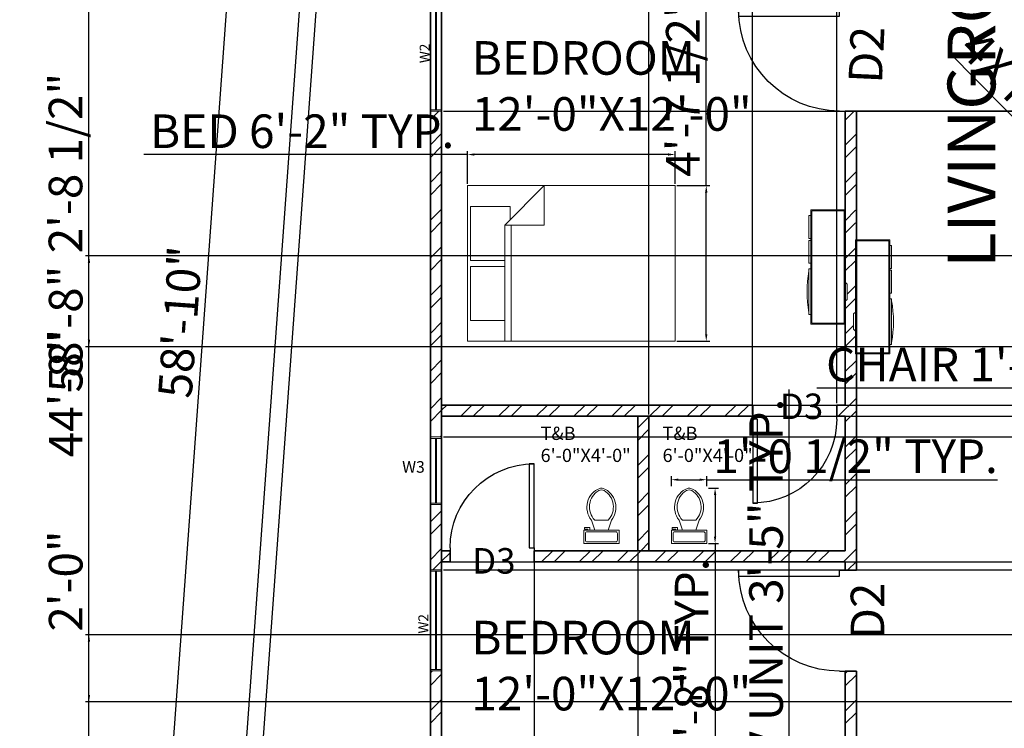
# Model space of a CAD drawing. Units: inches. Extents: x 2242 to 2870, y 1782 to 2635.
# Tile 2 of 7: x 2242 to 2594, y 2046 to 2299. Entities that reach past the tile are written whole.
import ezdxf

# ---------------------------------------------------------------- set-up
doc = ezdxf.new("R2010")
doc.units = ezdxf.units.IN
for name, color, linetype, lineweight in [('A-ANNO-DIMS', 7, 'Continuous', 18), ('A-ANNO-TEXT', 1, 'Continuous', 18), ('A-AREA-IDEN', 1, 'Continuous', 25), ('A-FLOR-FIXT', 9, 'Continuous', 18), ('A-WALL-PATT', 253, 'Continuous', 13), ('C-PROP', 7, 'Continuous', 30), ('doors', 5, 'Continuous', 25), ('furniture', 9, 'Continuous', 18), ('walls', 7, 'Continuous', 35), ('windows', 72, 'Continuous', 18)]:
    doc.layers.add(name, color=color, linetype=linetype, lineweight=lineweight)
doc.styles.get("Standard").update_dxf_attribs({"font": 'arial.ttf'})
doc.dimstyles.new('ISO-25', dxfattribs={"dimtxt": 12, "dimasz": 2.5, "dimexe": 1.25, "dimexo": 0.625, "dimtad": 1, "dimlunit": 4, "dimtxsty": 'Standard', "dimcen": 2.5, "dimadec": 0, "dimazin": 0, "dimtfac": 1, "dimtmove": 0, "dimatfit": 3, "dimfxl": 1, "dimarcsym": 0})

# ---------------------------------------------------------------- blocks, each defined once
blk = doc.blocks.new('*U2')
for p, q in [((0, 0), (0, -5)), ((30, 0), (30, -5))]:
    blk.add_line(p, q)
blk.add_lwpolyline([(0, 0), (0, 30), (1.75, 30), (1.75, 0)], close=True)
blk.add_arc((0, 0), 30, 0, 90)
blk = doc.blocks.new('Bed - Queen')
for p, q in [((0, -80.00003), (0, 0)), ((0, 0), (59.99999, 0)), ((59.99999, 0), (59.99999, -80.00003)), ((7.99999, -1.2), (28.79998, -1.2)), ((7.99999, -14.4), (7.99999, -1.2)), ((28.79998, -1.2), (28.79998, -14.4)), ((31.19999, -1.2), (51.99999, -1.2)), ((31.19999, -14.4), (31.19999, -1.2)), ((51.99999, -1.2), (51.99999, -16.4)), ((0, -14.4), (44.8, -14.4)), ((59.99999, -29.6), (44.8, -14.4)), ((44.8, -14.4), (44.8, -29.6)), ((44.8, -16.8), (0, -16.8)), ((51.99999, -16.4), (46.79936, -16.4)), ((44.8, -29.6), (59.99999, -29.6)), ((59.99999, -80.00003), (0, -80.00003))]:
    blk.add_line(p, q)
blk = doc.blocks.new('Toilet - top')
for p, q in [((9.5, -6), (9.5, -2)), ((-10, -8.5), (-8, -8.5)), ((-10, -9.5), (-10, -8.5)), ((-7, -9.5), (-10, -9.5)), ((-8, -8.5), (-8, -8)), ((-7, -8), (-7, -9.5)), ((-4, -8), (-6, -14)), ((4, -8), (6, -14)), ((4, -14), (-4, -14))]:
    blk.add_line(p, q)
blk.add_lwpolyline([(10.5, -8), (10.5, 0), (-10.5, 0), (-10.5, -8)], close=True)
for points in [[(-9.5, -2), (-9.5, -6)], [(8.5, -1), (-8.5, -1)], [(-8.5, -7), (8.5, -7)]]:
    blk.add_lwpolyline(points)
for centre, radius, start, end in [((-8.62, -1.88), 0.884, 81.8699, 188.1301), ((8.62, -1.88), 0.884, 351.8699, 98.1301), ((-8.62, -6.12), 0.884, 171.8699, 278.1301), ((8.62, -6.12), 0.884, 261.8699, 8.1301), ((3.52, -21.58), 12.17, 141.46911, 247.97143), ((4.2, -21.82), 11.33, 136.36773, 238.94682), ((-3.52, -21.58), 12.17, 292.02843, 38.53071), ((-4.2, -21.82), 11.33, 301.05301, 43.63209), ((0, -27.88), 4, 245.73182, 294.26817), ((0, -29), 4, 254.86053, 285.13947)]:
    blk.add_arc(centre, radius, start, end)
blk = doc.blocks.new('Entertainment Center')
for p, q in [((-4, 0), (-5, -1)), ((4, 0), (-4, 0)), ((5, -1), (4, 0)), ((-17, -19), (-17, -1)), ((-17, -1), (43, -1)), ((-16.5, -18.5), (-16.5, -1.5)), ((-16.5, -1.5), (42.5, -1.5)), ((42.5, -1.5), (42.5, -18.5)), ((43, -1), (43, -19)), ((43, -19), (-17, -19)), ((42.5, -18.5), (-16.5, -18.5)), ((-12, -20), (-12, -19)), ((12, -20), (-12, -20)), ((12, -19), (12, -20)), ((15, -20), (15, -19)), ((27, -20), (15, -20)), ((27, -19), (27, -20)), ((28, -20), (28, -19)), ((40, -20), (28, -20)), ((40, -19), (40, -20))]:
    blk.add_line(p, q)
blk.add_arc((0, 40), 61, 259.6111, 280.3889)
blk = doc.blocks.new('*D16')
at = {"layer": 'A-ANNO-DIMS', "color": 0, "lineweight": -2, "transparency": 16777216}
for p, q in [((2358.54, 2540.38), (2331.98, 2542.3)), ((2333.04, 2539.72), (2282.38, 1840.55)), ((2307.51, 1836.23), (2280.95, 1838.15))]:
    blk.add_line(p, q, dxfattribs=at)
at = {"layer": 'A-ANNO-DIMS', "color": 0, "transparency": 16777216}
for points in [[(2332.63, 2539.75), (2333.46, 2539.69), (2333.22, 2542.21)], [(2281.96, 1840.58), (2282.79, 1840.52), (2282.2, 1838.06)]]:
    blk.add_solid(points, dxfattribs=at)
at = {"layer": 'Defpoints', "color": 0, "transparency": 16777216}
for p in [(2359.16, 2540.33), (2282.2, 1838.06), (2308.14, 1836.18)]:
    blk.add_point(p, dxfattribs=at)
at = {"layer": 'A-ANNO-DIMS', "color": 0, "transparency": 16777216, "insert": (2300.98, 2190.63), "char_height": 12, "attachment_point": 5, "rotation": 85.8553}
blk.add_mtext('58\'-10"', dxfattribs=at)
blk = doc.blocks.new('WIN-W2-36IN')
for p, q in [((0, 4), (36.12, 4)), ((0, 0), (0, 4)), ((0.5, 0), (0.5, 4)), ((35.62, 4), (35.62, 0)), ((36.12, 4), (36.12, 0)), ((36.12, 0), (0, 0)), ((0.5, 2.2), (35.62, 2.2)), ((0.5, 1.8), (35.62, 1.8))]:
    blk.add_line(p, q)
blk = doc.blocks.new('WIN-W3-24IN')
for p, q in [((0, 0), (0, 24.12)), ((0, 24.12), (4, 24.12)), ((0, 23.62), (4, 23.62)), ((1.8, 23.62), (1.8, 0.5)), ((2.2, 23.62), (2.2, 0.5)), ((4, 24.12), (4, 0)), ((4, 0.5), (0, 0.5)), ((4, 0), (0, 0))]:
    blk.add_line(p, q)
blk = doc.blocks.new('*D39')
at = {"layer": 'A-ANNO-DIMS', "color": 0, "lineweight": -2, "transparency": 16777216}
for p, q in [((2401.96, 2250.56), (2286.47, 2250.56)), ((2401.96, 2240.07), (2401.96, 2251.81)), ((2473.56, 2250.56), (2404.46, 2250.56)), ((2476.06, 2240.07), (2476.06, 2251.81))]:
    blk.add_line(p, q, dxfattribs=at)
at = {"layer": 'A-ANNO-DIMS', "color": 0, "transparency": 16777216}
for points in [[(2404.46, 2250.98), (2404.46, 2250.15), (2401.96, 2250.56)], [(2473.56, 2250.98), (2473.56, 2250.15), (2476.06, 2250.56)]]:
    blk.add_solid(points, dxfattribs=at)
at = {"layer": 'Defpoints', "color": 0, "transparency": 16777216}
for p in [(2401.96, 2250.56), (2401.96, 2239.45), (2476.06, 2239.45)]:
    blk.add_point(p, dxfattribs=at)
at = {"layer": 'A-ANNO-DIMS', "color": 0, "transparency": 16777216, "insert": (2342.97, 2257.32), "char_height": 12, "attachment_point": 5}
blk.add_mtext('BED 6\'-2" TYP.', dxfattribs=at)
blk = doc.blocks.new('*D40')
at = {"layer": 'A-ANNO-DIMS', "color": 0, "lineweight": -2, "transparency": 16777216}
for p, q in [((2487.18, 2239.45), (2487.18, 2344.79)), ((2476.69, 2239.45), (2488.43, 2239.45)), ((2487.18, 2186.37), (2487.18, 2236.95)), ((2476.69, 2183.87), (2488.43, 2183.87))]:
    blk.add_line(p, q, dxfattribs=at)
at = {"layer": 'A-ANNO-DIMS', "color": 0, "transparency": 16777216}
for points in [[(2486.76, 2236.95), (2487.59, 2236.95), (2487.18, 2239.45)], [(2486.76, 2186.37), (2487.59, 2186.37), (2487.18, 2183.87)]]:
    blk.add_solid(points, dxfattribs=at)
at = {"layer": 'Defpoints', "color": 0, "transparency": 16777216}
for p in [(2476.06, 2239.45), (2487.18, 2239.45), (2476.06, 2183.87)]:
    blk.add_point(p, dxfattribs=at)
at = {"layer": 'A-ANNO-DIMS', "color": 0, "transparency": 16777216, "insert": (2480.35, 2293.37), "char_height": 12, "attachment_point": 5, "rotation": 90}
blk.add_mtext('4\'-7 1/2" TYP.', dxfattribs=at)
blk = doc.blocks.new('*D41')
at = {"layer": 'A-ANNO-DIMS', "color": 0, "lineweight": -2, "transparency": 16777216}
for p, q in [((2516.82, 2019.58), (2516.82, 2166.63)), ((2522.31, 2019.58), (2515.57, 2019.58)), ((2516.82, 1981.32), (2516.82, 2017.08)), ((2522.31, 1978.82), (2515.57, 1978.82))]:
    blk.add_line(p, q, dxfattribs=at)
at = {"layer": 'A-ANNO-DIMS', "color": 0, "transparency": 16777216}
for points in [[(2516.4, 2017.08), (2517.23, 2017.08), (2516.82, 2019.58)], [(2516.4, 1981.32), (2517.23, 1981.32), (2516.82, 1978.82)]]:
    blk.add_solid(points, dxfattribs=at)
at = {"layer": 'Defpoints', "color": 0, "transparency": 16777216}
for p in [(2516.82, 2019.58), (2522.93, 2019.58), (2522.93, 1978.82)]:
    blk.add_point(p, dxfattribs=at)
at = {"layer": 'A-ANNO-DIMS', "color": 0, "transparency": 16777216, "insert": (2510.06, 2094.35), "char_height": 12, "attachment_point": 5, "rotation": 90}
blk.add_mtext('TV UNIT 3\'-5" TYP.', dxfattribs=at)
blk = doc.blocks.new('*D42')
at = {"layer": 'A-ANNO-DIMS', "color": 0, "lineweight": -2, "transparency": 16777216}
for p, q in [((2522.93, 2020.21), (2522.93, 2026.94)), ((2525.43, 2025.69), (2534.92, 2025.69)), ((2537.42, 2020.21), (2537.42, 2026.94)), ((2537.42, 2025.69), (2641.15, 2025.69))]:
    blk.add_line(p, q, dxfattribs=at)
at = {"layer": 'A-ANNO-DIMS', "color": 0, "transparency": 16777216}
for points in [[(2525.43, 2026.11), (2525.43, 2025.28), (2522.93, 2025.69)], [(2534.92, 2026.11), (2534.92, 2025.28), (2537.42, 2025.69)]]:
    blk.add_solid(points, dxfattribs=at)
at = {"layer": 'Defpoints', "color": 0, "transparency": 16777216}
for p in [(2537.42, 2025.69), (2522.93, 2019.58), (2537.42, 2019.58)]:
    blk.add_point(p, dxfattribs=at)
at = {"layer": 'A-ANNO-DIMS', "color": 0, "transparency": 16777216, "insert": (2590.54, 2032.52), "char_height": 12, "attachment_point": 5}
blk.add_mtext('1\'-2 1/2" TYP.', dxfattribs=at)
blk = doc.blocks.new('*D43')
at = {"layer": 'A-ANNO-DIMS', "color": 0, "lineweight": -2, "transparency": 16777216}
for p, q in [((2660.19, 2165.56), (2660.19, 2168.42)), ((2675.05, 2165.56), (2675.05, 2168.42)), ((2660.19, 2167.17), (2526.62, 2167.17)), ((2672.55, 2167.17), (2662.69, 2167.17))]:
    blk.add_line(p, q, dxfattribs=at)
at = {"layer": 'A-ANNO-DIMS', "color": 0, "transparency": 16777216}
for points in [[(2662.69, 2167.59), (2662.69, 2166.75), (2660.19, 2167.17)], [(2672.55, 2167.59), (2672.55, 2166.75), (2675.05, 2167.17)]]:
    blk.add_solid(points, dxfattribs=at)
at = {"layer": 'Defpoints', "color": 0, "transparency": 16777216}
for p in [(2660.19, 2167.17), (2660.19, 2164.94), (2675.05, 2164.94)]:
    blk.add_point(p, dxfattribs=at)
at = {"layer": 'A-ANNO-DIMS', "color": 0, "transparency": 16777216, "insert": (2592.15, 2174), "char_height": 12, "attachment_point": 5}
blk.add_mtext('CHAIR 1\'-3" TYP.', dxfattribs=at)
blk = doc.blocks.new('*D49')
at = {"layer": 'A-ANNO-DIMS', "color": 0, "lineweight": -2, "transparency": 16777216}
for p, q in [((2487.98, 2131.46), (2491.58, 2131.46)), ((2490.33, 2128.96), (2490.33, 2114.14)), ((2487.98, 2111.64), (2491.58, 2111.64)), ((2490.33, 2111.64), (2490.33, 2001.67))]:
    blk.add_line(p, q, dxfattribs=at)
at = {"layer": 'A-ANNO-DIMS', "color": 0, "transparency": 16777216}
for points in [[(2489.91, 2128.96), (2490.75, 2128.96), (2490.33, 2131.46)], [(2489.91, 2114.14), (2490.75, 2114.14), (2490.33, 2111.64)]]:
    blk.add_solid(points, dxfattribs=at)
at = {"layer": 'Defpoints', "color": 0, "transparency": 16777216}
for p in [(2487.36, 2131.46), (2487.36, 2111.64), (2490.33, 2111.64)]:
    blk.add_point(p, dxfattribs=at)
at = {"layer": 'A-ANNO-DIMS', "color": 0, "transparency": 16777216, "insert": (2483.5, 2055.41), "char_height": 12, "attachment_point": 5, "rotation": 90}
blk.add_mtext('WC 1\'-8" TYP.', dxfattribs=at)
blk = doc.blocks.new('*D50')
at = {"layer": 'A-ANNO-DIMS', "color": 0, "lineweight": -2, "transparency": 16777216}
for p, q in [((2474.76, 2132.09), (2474.76, 2135.68)), ((2477.26, 2134.43), (2484.86, 2134.43)), ((2487.36, 2132.09), (2487.36, 2135.68)), ((2487.36, 2134.43), (2591.08, 2134.43))]:
    blk.add_line(p, q, dxfattribs=at)
at = {"layer": 'A-ANNO-DIMS', "color": 0, "transparency": 16777216}
for points in [[(2477.26, 2134.85), (2477.26, 2134.02), (2474.76, 2134.43)], [(2484.86, 2134.85), (2484.86, 2134.02), (2487.36, 2134.43)]]:
    blk.add_solid(points, dxfattribs=at)
at = {"layer": 'Defpoints', "color": 0, "transparency": 16777216}
for p in [(2487.36, 2134.43), (2474.76, 2131.46), (2487.36, 2131.46)]:
    blk.add_point(p, dxfattribs=at)
at = {"layer": 'A-ANNO-DIMS', "color": 0, "transparency": 16777216, "insert": (2540.47, 2141.26), "char_height": 12, "attachment_point": 5}
blk.add_mtext('1\'-0 1/2" TYP.', dxfattribs=at)
blk = doc.blocks.new('*D55')
at = {"layer": 'A-ANNO-DIMS', "color": 0, "lineweight": -2, "transparency": 16777216}
for p, q in [((2358.54, 2540.33), (2265.64, 2540.33)), ((2266.89, 1838.68), (2266.89, 2537.83)), ((2307.51, 1836.18), (2265.64, 1836.18))]:
    blk.add_line(p, q, dxfattribs=at)
at = {"layer": 'A-ANNO-DIMS', "color": 0, "transparency": 16777216}
for points in [[(2266.47, 2537.83), (2267.3, 2537.83), (2266.89, 2540.33)], [(2266.47, 1838.68), (2267.3, 1838.68), (2266.89, 1836.18)]]:
    blk.add_solid(points, dxfattribs=at)
at = {"layer": 'Defpoints', "color": 0, "transparency": 16777216}
for p in [(2266.89, 2540.33), (2359.16, 2540.33), (2308.14, 1836.18)]:
    blk.add_point(p, dxfattribs=at)
at = {"layer": 'A-ANNO-DIMS', "color": 0, "transparency": 16777216, "insert": (2260.13, 2188.26), "char_height": 12, "attachment_point": 5, "rotation": 90}
blk.add_mtext('58\'-8"', dxfattribs=at)
blk = doc.blocks.new('*D58')
at = {"layer": 'A-ANNO-DIMS', "color": 0, "lineweight": -2, "transparency": 16777216}
for p, q in [((2388.12, 2433.1), (2265.64, 2433.1)), ((2266.89, 1899.6), (2266.89, 2430.6)), ((2388.12, 1897.1), (2265.64, 1897.1))]:
    blk.add_line(p, q, dxfattribs=at)
at = {"layer": 'A-ANNO-DIMS', "color": 0, "transparency": 16777216}
for points in [[(2266.47, 2430.6), (2267.3, 2430.6), (2266.89, 2433.1)], [(2266.47, 1899.6), (2267.3, 1899.6), (2266.89, 1897.1)]]:
    blk.add_solid(points, dxfattribs=at)
at = {"layer": 'Defpoints', "color": 0, "transparency": 16777216}
for p in [(2266.89, 2433.1), (2388.74, 2433.1), (2388.74, 1897.1)]:
    blk.add_point(p, dxfattribs=at)
at = {"layer": 'A-ANNO-DIMS', "color": 0, "transparency": 16777216, "insert": (2260.13, 2165.1), "char_height": 12, "attachment_point": 5, "rotation": 90}
blk.add_mtext('44\'-8"', dxfattribs=at)
blk = doc.blocks.new('*D62')
at = {"layer": 'A-ANNO-DIMS', "color": 0, "lineweight": -2, "transparency": 16777216}
for p, q in [((2537.37, 2302.1), (2797.66, 2302.1)), ((2796.41, 2299.6), (2796.41, 2268.6)), ((2537.37, 2266.1), (2797.66, 2266.1))]:
    blk.add_line(p, q, dxfattribs=at)
at = {"layer": 'A-ANNO-DIMS', "color": 0, "transparency": 16777216}
for points in [[(2796, 2299.6), (2796.83, 2299.6), (2796.41, 2302.1)], [(2796, 2268.6), (2796.83, 2268.6), (2796.41, 2266.1)]]:
    blk.add_solid(points, dxfattribs=at)
at = {"layer": 'Defpoints', "color": 0, "transparency": 16777216}
for p in [(2536.74, 2302.1), (2536.74, 2266.1), (2796.41, 2266.1)]:
    blk.add_point(p, dxfattribs=at)
at = {"layer": 'A-ANNO-DIMS', "color": 0, "transparency": 16777216, "insert": (2789.66, 2284.1), "char_height": 12, "attachment_point": 5, "rotation": 90}
blk.add_mtext('3\'-0"', dxfattribs=at)
blk = doc.blocks.new('*D63')
at = {"layer": 'A-ANNO-DIMS', "color": 0, "lineweight": -2, "transparency": 16777216}
for p, q in [((2503.74, 2161.72), (2503.74, 2611.83)), ((2533.74, 2161.72), (2533.74, 2611.83)), ((2506.24, 2610.58), (2531.24, 2610.58)), ((2533.74, 2610.58), (2569.6, 2610.58))]:
    blk.add_line(p, q, dxfattribs=at)
at = {"layer": 'A-ANNO-DIMS', "color": 0, "transparency": 16777216}
for points in [[(2506.24, 2611), (2506.24, 2610.17), (2503.74, 2610.58)], [(2531.24, 2611), (2531.24, 2610.17), (2533.74, 2610.58)]]:
    blk.add_solid(points, dxfattribs=at)
at = {"layer": 'Defpoints', "color": 0, "transparency": 16777216}
for p in [(2533.74, 2610.58), (2503.74, 2161.1), (2533.74, 2161.1)]:
    blk.add_point(p, dxfattribs=at)
at = {"layer": 'A-ANNO-DIMS', "color": 0, "transparency": 16777216, "insert": (2552.92, 2617.34), "char_height": 12, "attachment_point": 5}
blk.add_mtext('2\'-6"', dxfattribs=at)
blk = doc.blocks.new('*D75')
at = {"layer": 'A-ANNO-DIMS', "color": 0, "lineweight": -2, "transparency": 16777216}
for p, q in [((2266.89, 2214.36), (2266.89, 2278.18)), ((2651.13, 2214.36), (2265.64, 2214.36)), ((2266.89, 2184.4), (2266.89, 2211.86)), ((2651.13, 2181.9), (2265.64, 2181.9))]:
    blk.add_line(p, q, dxfattribs=at)
at = {"layer": 'A-ANNO-DIMS', "color": 0, "transparency": 16777216}
for points in [[(2266.47, 2211.86), (2267.3, 2211.86), (2266.89, 2214.36)], [(2266.47, 2184.4), (2267.3, 2184.4), (2266.89, 2181.9)]]:
    blk.add_solid(points, dxfattribs=at)
at = {"layer": 'Defpoints', "color": 0, "transparency": 16777216}
for p in [(2266.89, 2214.36), (2651.75, 2214.36), (2651.75, 2181.9)]:
    blk.add_point(p, dxfattribs=at)
at = {"layer": 'A-ANNO-DIMS', "color": 0, "transparency": 16777216, "insert": (2260.06, 2247.52), "char_height": 12, "attachment_point": 5, "rotation": 90}
blk.add_mtext('2\'-8 1/2"', dxfattribs=at)
blk = doc.blocks.new('*D77')
at = {"layer": 'A-ANNO-DIMS', "color": 0, "lineweight": -2, "transparency": 16777216}
for p, q in [((2393.37, 2157.1), (2797.66, 2157.1)), ((2796.41, 2154.6), (2796.41, 2152.19)), ((2393.37, 2149.69), (2797.66, 2149.69)), ((2796.41, 2149.69), (2796.41, 2086.08))]:
    blk.add_line(p, q, dxfattribs=at)
at = {"layer": 'A-ANNO-DIMS', "color": 0, "transparency": 16777216}
for points in [[(2796, 2154.6), (2796.83, 2154.6), (2796.41, 2157.1)], [(2796, 2152.19), (2796.83, 2152.19), (2796.41, 2149.69)]]:
    blk.add_solid(points, dxfattribs=at)
at = {"layer": 'Defpoints', "color": 0, "transparency": 16777216}
for p in [(2392.74, 2157.1), (2392.74, 2149.69), (2796.41, 2149.69)]:
    blk.add_point(p, dxfattribs=at)
at = {"layer": 'A-ANNO-DIMS', "color": 0, "transparency": 16777216, "insert": (2789.58, 2116.64), "char_height": 12, "attachment_point": 5, "rotation": 90}
blk.add_mtext('0\'-7 1/2"', dxfattribs=at)
blk = doc.blocks.new('*D78')
at = {"layer": 'A-ANNO-DIMS', "color": 0, "lineweight": -2, "transparency": 16777216}
for p, q in [((2796.41, 2107.6), (2796.41, 2110.1)), ((2393.37, 2105.1), (2797.66, 2105.1)), ((2796.41, 2105.1), (2796.41, 2102.29)), ((2393.37, 2102.29), (2797.66, 2102.29)), ((2796.41, 2099.79), (2796.41, 2064.14))]:
    blk.add_line(p, q, dxfattribs=at)
at = {"layer": 'A-ANNO-DIMS', "color": 0, "transparency": 16777216}
for points in [[(2796, 2107.6), (2796.83, 2107.6), (2796.41, 2105.1)], [(2796, 2099.79), (2796.83, 2099.79), (2796.41, 2102.29)]]:
    blk.add_solid(points, dxfattribs=at)
at = {"layer": 'Defpoints', "color": 0, "transparency": 16777216}
for p in [(2392.74, 2105.1), (2392.74, 2102.29), (2796.41, 2102.29)]:
    blk.add_point(p, dxfattribs=at)
at = {"layer": 'A-ANNO-DIMS', "color": 0, "transparency": 16777216, "insert": (2789.66, 2080.72), "char_height": 12, "attachment_point": 5, "rotation": 90}
blk.add_mtext('0\'-3"', dxfattribs=at)
blk = doc.blocks.new('*D80')
at = {"layer": 'A-ANNO-DIMS', "color": 0, "lineweight": -2, "transparency": 16777216}
for p, q in [((2393.37, 2265.99), (2797.66, 2265.99)), ((2796.41, 2163.6), (2796.41, 2263.49)), ((2393.37, 2161.1), (2797.66, 2161.1))]:
    blk.add_line(p, q, dxfattribs=at)
at = {"layer": 'A-ANNO-DIMS', "color": 0, "transparency": 16777216}
for points in [[(2796, 2263.49), (2796.83, 2263.49), (2796.41, 2265.99)], [(2796, 2163.6), (2796.83, 2163.6), (2796.41, 2161.1)]]:
    blk.add_solid(points, dxfattribs=at)
at = {"layer": 'Defpoints', "color": 0, "transparency": 16777216}
for p in [(2392.74, 2265.99), (2796.41, 2265.99), (2392.74, 2161.1)]:
    blk.add_point(p, dxfattribs=at)
at = {"layer": 'A-ANNO-DIMS', "color": 0, "transparency": 16777216, "insert": (2789.66, 2213.55), "char_height": 12, "attachment_point": 5, "rotation": 90}
blk.add_mtext('8\'-9"', dxfattribs=at)
blk = doc.blocks.new('*D81')
at = {"layer": 'A-ANNO-DIMS', "color": 0, "lineweight": -2, "transparency": 16777216}
for p, q in [((2266.89, 2079.1), (2266.89, 2114.95)), ((2672.54, 2079.1), (2265.64, 2079.1)), ((2266.89, 2057.6), (2266.89, 2076.6)), ((2672.54, 2055.1), (2265.64, 2055.1))]:
    blk.add_line(p, q, dxfattribs=at)
at = {"layer": 'A-ANNO-DIMS', "color": 0, "transparency": 16777216}
for points in [[(2266.47, 2076.6), (2267.3, 2076.6), (2266.89, 2079.1)], [(2266.47, 2057.6), (2267.3, 2057.6), (2266.89, 2055.1)]]:
    blk.add_solid(points, dxfattribs=at)
at = {"layer": 'Defpoints', "color": 0, "transparency": 16777216}
for p in [(2266.89, 2079.1), (2673.16, 2079.1), (2673.16, 2055.1)]:
    blk.add_point(p, dxfattribs=at)
at = {"layer": 'A-ANNO-DIMS', "color": 0, "transparency": 16777216, "insert": (2260.13, 2098.27), "char_height": 12, "attachment_point": 5, "rotation": 90}
blk.add_mtext('2\'-0"', dxfattribs=at)
blk = doc.blocks.new('*D86')
at = {"layer": 'A-ANNO-DIMS', "color": 0, "lineweight": -2, "transparency": 16777216}
for p, q in [((2425.74, 2108.47), (2425.74, 1793.68)), ((2462.74, 2108.47), (2462.74, 1793.68)), ((2428.24, 1794.93), (2460.24, 1794.93))]:
    blk.add_line(p, q, dxfattribs=at)
at = {"layer": 'A-ANNO-DIMS', "color": 0, "transparency": 16777216}
for points in [[(2428.24, 1795.35), (2428.24, 1794.51), (2425.74, 1794.93)], [(2460.24, 1795.35), (2460.24, 1794.51), (2462.74, 1794.93)]]:
    blk.add_solid(points, dxfattribs=at)
at = {"layer": 'Defpoints', "color": 0, "transparency": 16777216}
for p in [(2425.74, 2109.1), (2462.74, 2109.1), (2462.74, 1794.93)]:
    blk.add_point(p, dxfattribs=at)
at = {"layer": 'A-ANNO-DIMS', "color": 0, "transparency": 16777216, "insert": (2444.24, 1801.69), "char_height": 12, "attachment_point": 5}
blk.add_mtext('3\'-1"', dxfattribs=at)
blk = doc.blocks.new('*D87')
at = {"layer": 'A-ANNO-DIMS', "color": 0, "lineweight": -2, "transparency": 16777216}
for p, q in [((2466.74, 2157.72), (2466.74, 2611.83)), ((2503.74, 2157.72), (2503.74, 2611.83)), ((2469.24, 2610.58), (2501.24, 2610.58))]:
    blk.add_line(p, q, dxfattribs=at)
at = {"layer": 'A-ANNO-DIMS', "color": 0, "transparency": 16777216}
for points in [[(2469.24, 2611), (2469.24, 2610.17), (2466.74, 2610.58)], [(2501.24, 2611), (2501.24, 2610.17), (2503.74, 2610.58)]]:
    blk.add_solid(points, dxfattribs=at)
at = {"layer": 'Defpoints', "color": 0, "transparency": 16777216}
for p in [(2503.74, 2610.58), (2466.74, 2157.1), (2503.74, 2157.1)]:
    blk.add_point(p, dxfattribs=at)
at = {"layer": 'A-ANNO-DIMS', "color": 0, "transparency": 16777216, "insert": (2485.24, 2617.34), "char_height": 12, "attachment_point": 5}
blk.add_mtext('3\'-1"', dxfattribs=at)
blk = doc.blocks.new('*D88')
at = {"layer": 'A-ANNO-DIMS', "color": 0, "lineweight": -2, "transparency": 16777216}
for p, q in [((2574.38, 2286.56), (2645.45, 2214.28)), ((2651.75, 2207.87), (2647.2, 2212.5))]:
    blk.add_line(p, q, dxfattribs=at)
at = {"layer": 'A-ANNO-DIMS', "color": 0, "transparency": 16777216}
blk.add_solid([(2645.74, 2214.58), (2645.15, 2213.99), (2647.2, 2212.5)], dxfattribs=at)
at = {"layer": 'Defpoints', "color": 0, "transparency": 16777216}
for p in [(2647.2, 2212.5), (2651.75, 2207.87)]:
    blk.add_point(p, dxfattribs=at)
at = {"layer": 'A-ANNO-DIMS', "color": 0, "transparency": 16777216, "insert": (2613.91, 2256.1), "char_height": 12, "attachment_point": 5, "rotation": 314.5145}
blk.add_mtext('4X R0\'-6 1/2"', dxfattribs=at)

msp = doc.modelspace()

# ---------------------------------------------------------------- hatches: boundary and pattern name
at = {"layer": 'A-WALL-PATT'}
h = msp.add_hatch(dxfattribs=at)
h.set_pattern_fill('ANSI32', color=256)
h.paths.add_polyline_path([(2392.745, 2265.993), (2388.745, 2265.993), (2388.745, 2149.693), (2392.745, 2149.693)])
h = msp.add_hatch(dxfattribs=at)
h.set_pattern_fill('ANSI32', color=256)
h.paths.add_polyline_path([(2540.405, 2220.104), (2540.745, 2266.097), (2536.745, 2266.097), (2536.745, 2204.961), (2537.424, 2204.281), (2537.424, 2198.847), (2536.745, 2198.167), (2536.745, 2190.015), (2536.745, 2161.097), (2533.745, 2161.097), (2533.745, 2157.097), (2536.745, 2157.097), (2536.745, 2109.097), (2425.745, 2109.097), (2425.745, 2105.097), (2536.745, 2105.097), (2536.745, 2102.097), (2540.745, 2102.097), (2540.745, 2105.097), (2540.745, 2179.344), (2540.405, 2179.344), (2540.405, 2187.496), (2539.726, 2188.175), (2539.726, 2193.61), (2540.405, 2194.29)])
h = msp.add_hatch(dxfattribs=at)
h.set_pattern_fill('ANSI32', color=256)
h.paths.add_polyline_path([(2503.745, 2161.097), (2392.745, 2161.097), (2392.745, 2157.097), (2503.745, 2157.097)])
h = msp.add_hatch(dxfattribs=at)
h.set_pattern_fill('ANSI32', color=256)
h.paths.add_polyline_path([(2466.745, 2157.097), (2462.745, 2157.097), (2462.745, 2109.097), (2466.745, 2109.097)], flags=17)
h = msp.add_hatch(dxfattribs=at)
h.set_pattern_fill('ANSI32', color=256)
h.paths.add_polyline_path([(2392.745, 2125.577), (2388.745, 2125.577), (2388.745, 2102.29), (2392.745, 2102.29)])
h = msp.add_hatch(dxfattribs=at)
h.set_pattern_fill('ANSI32', color=256)
h.paths.add_polyline_path([(2395.745, 2109.097), (2392.745, 2109.097), (2392.745, 2105.097), (2395.745, 2105.097)])
h = msp.add_hatch(dxfattribs=at)
h.set_pattern_fill('ANSI32', color=256)
h.paths.add_polyline_path([(2392.745, 2066.174), (2388.745, 2066.174), (2388.745, 1957.097), (2484.674, 1957.097), (2484.674, 1961.097), (2392.745, 1961.097)])
h = msp.add_hatch(dxfattribs=at)
h.set_pattern_fill('ANSI32', color=256)
h.paths.add_polyline_path([(2540.745, 2066.097), (2536.745, 2066.097), (2536.745, 1993.766), (2537.424, 1993.086), (2537.424, 1987.651), (2536.745, 1986.972), (2536.745, 1978.82), (2536.745, 1961.097), (2540.745, 1961.097)])

# ---------------------------------------------------------------- linework, layer by layer
at = {"layer": 'C-PROP'}
for p, q in [((2359.164, 2540.335), (2308.137, 1836.181)), ((2364.745, 2534.335), (2314.71, 1843.873))]:
    msp.add_line(p, q, dxfattribs=at)
at = {"layer": 'walls'}
for p, q in [((2388.745, 1957.097), (2388.745, 2433.097)), ((2392.745, 1961.097), (2392.745, 2429.097)), ((2536.745, 2266.097), (2540.745, 2266.097)), ((2536.745, 2161.097), (2536.745, 2266.097)), ((2540.745, 2102.097), (2540.745, 2266.097)), ((2503.745, 2161.097), (2392.745, 2161.097)), ((2503.745, 2161.097), (2503.745, 2157.097)), ((2536.745, 2161.097), (2533.745, 2161.097)), ((2533.745, 2157.097), (2533.745, 2161.097)), ((2503.745, 2157.097), (2392.745, 2157.097)), ((2462.745, 2109.097), (2462.745, 2157.097)), ((2466.745, 2109.097), (2466.745, 2157.097)), ((2536.745, 2157.097), (2533.745, 2157.097)), ((2536.745, 2157.097), (2533.745, 2157.097)), ((2536.745, 2109.097), (2536.745, 2157.097)), ((2395.745, 2109.097), (2392.745, 2109.097)), ((2395.745, 2105.097), (2395.745, 2109.097)), ((2536.745, 2109.097), (2425.745, 2109.097)), ((2425.745, 2109.097), (2425.745, 2105.097)), ((2392.745, 2105.097), (2395.745, 2105.097)), ((2395.745, 2105.097), (2392.745, 2105.097)), ((2536.745, 2105.097), (2425.745, 2105.097)), ((2536.745, 2102.097), (2536.745, 2105.097)), ((2540.745, 2105.097), (2540.745, 2102.097)), ((2540.745, 2102.097), (2536.745, 2102.097)), ((2536.745, 1961.097), (2536.745, 2066.097)), ((2536.745, 2066.097), (2540.745, 2066.097)), ((2540.745, 1961.097), (2540.745, 2066.097))]:
    msp.add_line(p, q, dxfattribs=at)

# ---------------------------------------------------------------- block references
at = {"layer": 'A-FLOR-FIXT', "xscale": -0.5996549294202672, "yscale": 0.5996549294202672, "zscale": 0.5996549294202672, "rotation": 180}
for p in [(2449.77, 2111.645), (2481.06, 2111.645)]:
    msp.add_blockref('Toilet - top', p, dxfattribs=at)
at = {"layer": 'doors', "xscale": -1.199999999999999, "yscale": 1.199999999999999, "zscale": 1.199999999999999, "rotation": 90}
for p in [(2534.745, 2302.097), (2534.745, 2102.097)]:
    msp.add_blockref('*U2', p, dxfattribs=at)
at = {"layer": 'doors', "xscale": -1, "rotation": 180}
msp.add_blockref('*U2', (2503.745, 2156.097), dxfattribs=at)
at = {"layer": 'doors', "xscale": -1}
msp.add_blockref('*U2', (2425.745, 2110.097), dxfattribs=at)
at = {"layer": 'furniture'}
for name, p, xscale, yscale, zscale, rotation in [('Bed - Queen', (2401.963, 2183.874), 0.9262549739508827, 0.9262549739508827, 0.9262549739508827, 90), ('Entertainment Center', (2537.424, 2201.564), -0.6793374069686555, 0.6793374069686555, 0.6793374069686555, 270), ('Entertainment Center', (2539.726, 2190.893), 0.6793374069686555, 0.6793374069686555, 0.6793374069686555, 90)]:
    msp.add_blockref(name, p, dxfattribs=dict(at, xscale=xscale, yscale=yscale, zscale=zscale, rotation=rotation))
at = {"layer": 'windows', "rotation": 89.99999999999604}
for p in [(2392.745, 2265.993), (2392.745, 2066.174)]:
    msp.add_blockref('WIN-W2-36IN', p, dxfattribs=at)
at = {"layer": 'windows'}
msp.add_blockref('WIN-W3-24IN', (2388.745, 2125.577), dxfattribs=at)

# ---------------------------------------------------------------- texts
at = {"layer": 'A-ANNO-TEXT', "attachment_point": 1}
for s, width, gutter_width, insert, char_height, rotation in [('D2', 2.16795, 12.5, (2537.887, 2276.305), 12, 87.35661), ('W2', 0.34623, 17.788, (2384.903, 2283.192), 3.5576, 90), ('D2', 2.16795, 12.5, (2538.722, 2077.336), 12, 90), ('W2', 0.34623, 17.788, (2384.446, 2079.496), 3.5576, 90)]:
    msp.add_mtext_dynamic_manual_height_columns(s, width=width, gutter_width=gutter_width, heights=[0], dxfattribs=dict(at, insert=insert, char_height=char_height, rotation=rotation))
for s, width, gutter_width, insert, char_height in [('D3', 1.64651, 9.493, (2513.458, 2165.203), 9.1137), ('W3', 1.14454, 20.658, (2378.657, 2141.061), 4.1316), ('D3', 1.64651, 9.493, (2403.643, 2110.016), 9.1137)]:
    msp.add_mtext_dynamic_manual_height_columns(s, width=width, gutter_width=gutter_width, heights=[0], dxfattribs=dict(at, insert=insert, char_height=char_height))
at = {"layer": 'A-AREA-IDEN', "insert": (2573.308, 2210.091), "char_height": 17.04609, "attachment_point": 1, "rotation": 90}
msp.add_mtext_dynamic_manual_height_columns('LIVINGROOM\\P14\'-3"X27\'-3"', width=6.2214, gutter_width=17.756, heights=[0], dxfattribs=at)
at = {"layer": 'A-AREA-IDEN', "attachment_point": 1}
for s, width, gutter_width, insert, char_height in [('BEDROOM\\P12\'-0"X12\'-0"', 4.3797, 12.5, (2403.518, 2291.044), 12), ('T&B\\P6\'-0"X4\'-0"', 0.50549, 23.61, (2428.062, 2153.358), 4.72198), ('T&B\\P6\'-0"X4\'-0"', 0.50549, 23.61, (2471.58, 2153.358), 4.72198), ('BEDROOM\\P12\'-0"X12\'-0"', 4.3797, 12.5, (2403.37, 2084.056), 12)]:
    msp.add_mtext_dynamic_manual_height_columns(s, width=width, gutter_width=gutter_width, heights=[0], dxfattribs=dict(at, insert=insert, char_height=char_height))

# ---------------------------------------------------------------- dimensions: what is measured, and where the dimension line sits
at = {"layer": 'A-ANNO-DIMS'}
for base, p1, p2, picture, middle in [((2503.745, 2610.585), (2466.745, 2157.097), (2503.745, 2157.097), '*D87', (2485.245, 2617.341)), ((2533.745, 2610.585), (2503.745, 2161.097), (2533.745, 2161.097), '*D63', (2552.921, 2617.337)), ((2462.745, 1794.931), (2425.745, 2109.097), (2462.745, 2109.097), '*D86', (2444.245, 1801.687))]:
    dim = msp.add_linear_dim(base=base, p1=p1, p2=p2, dimstyle='ISO-25', override={"dimdec": 1, "dimlfac": 1, "dimrnd": 0, "dimzin": 1, "dimdsep": 46, "dimlunit": 4, "dimfrac": 2}, dxfattribs=at)
    dim.commit()
    dim.dimension.update_dxf_attribs({"geometry": picture, "text_midpoint": middle})
dim = msp.add_aligned_dim(p1=(2359.164, 2540.335), p2=(2308.137, 1836.181), distance=-26.007, dimstyle='ISO-25', override={"dimclrd": 0, "dimclre": 0, "dimclrt": 0}, dxfattribs=at)
dim.commit()
dim.dimension.update_dxf_attribs({"geometry": '*D16', "text_midpoint": (2300.976, 2190.626)})
for base, p1, p2, picture, middle in [((2266.887, 2540.335), (2308.137, 1836.181), (2359.164, 2540.335), '*D55', (2260.135, 2188.258)), ((2266.887, 2433.097), (2388.745, 1897.097), (2388.745, 2433.097), '*D58', (2260.135, 2165.097)), ((2796.414, 2266.097), (2536.745, 2302.097), (2536.745, 2266.097), '*D62', (2789.658, 2284.097)), ((2266.887, 2214.364), (2651.751, 2181.899), (2651.751, 2214.364), '*D75', (2260.057, 2247.522)), ((2796.414, 2265.993), (2392.745, 2161.097), (2392.745, 2265.993), '*D80', (2789.662, 2213.545)), ((2796.414, 2149.693), (2392.745, 2157.097), (2392.745, 2149.693), '*D77', (2789.584, 2116.638)), ((2266.887, 2079.097), (2673.164, 2055.097), (2673.164, 2079.097), '*D81', (2260.135, 2098.274)), ((2796.414, 2102.29), (2392.745, 2105.097), (2392.745, 2102.29), '*D78', (2789.658, 2080.716))]:
    dim = msp.add_linear_dim(base=base, p1=p1, p2=p2, angle=90, dimstyle='ISO-25', override={"dimdec": 1, "dimlfac": 1, "dimrnd": 0, "dimzin": 1, "dimdsep": 46, "dimlunit": 4, "dimfrac": 2}, dxfattribs=at)
    dim.commit()
    dim.dimension.update_dxf_attribs({"geometry": picture, "text_midpoint": middle})
for base, p1, p2, angle, text, picture, middle in [((2487.178, 2239.449), (2476.063, 2183.874), (2476.063, 2239.449), 90, '<> TYP.', '*D40', (2480.349, 2293.369)), ((2401.963, 2250.564), (2476.063, 2239.449), (2401.963, 2239.449), 180, 'BED <> TYP.', '*D39', (2342.967, 2257.316)), ((2660.189, 2167.169), (2675.051, 2164.94), (2660.189, 2164.94), 180, 'CHAIR <> TYP.', '*D43', (2592.152, 2174.003)), ((2516.817, 2019.58), (2522.931, 1978.82), (2522.931, 2019.58), 90, 'TV UNIT <> TYP.', '*D41', (2510.061, 2094.353)), ((2490.328, 2111.645), (2487.356, 2131.461), (2487.356, 2111.645), 270, 'WC <> TYP.', '*D49', (2483.499, 2055.408))]:
    dim = msp.add_linear_dim(base=base, p1=p1, p2=p2, angle=angle, text=text, dimstyle='ISO-25', override={"dimdec": 1, "dimlfac": 1, "dimrnd": 0, "dimzin": 1, "dimdsep": 46, "dimlunit": 4, "dimfrac": 2}, dxfattribs=at)
    dim.commit()
    dim.dimension.update_dxf_attribs({"geometry": picture, "text_midpoint": middle})
dim = msp.add_radius_dim(center=(2651.751, 2207.871), mpoint=(2647.199, 2212.501), text='4X <>', dimstyle='ISO-25', override={"dimdec": 1, "dimlfac": 1, "dimrnd": 0, "dimzin": 1, "dimdsep": 46, "dimlunit": 4, "dimfrac": 2}, dxfattribs=at)
dim.commit()
dim.dimension.update_dxf_attribs({"geometry": '*D88', "text_midpoint": (2613.908, 2256.103)})
for base, p1, p2, picture, middle in [((2487.356, 2134.434), (2474.763, 2131.461), (2487.356, 2131.461), '*D50', (2540.47, 2141.263)), ((2537.424, 2025.694), (2522.931, 2019.58), (2537.424, 2019.58), '*D42', (2590.538, 2032.524))]:
    dim = msp.add_linear_dim(base=base, p1=p1, p2=p2, text='<> TYP.', dimstyle='ISO-25', override={"dimdec": 1, "dimlfac": 1, "dimrnd": 0, "dimzin": 1, "dimdsep": 46, "dimlunit": 4, "dimfrac": 2}, dxfattribs=at)
    dim.commit()
    dim.dimension.update_dxf_attribs({"geometry": picture, "text_midpoint": middle})

doc.saveas('drawing.dxf')
